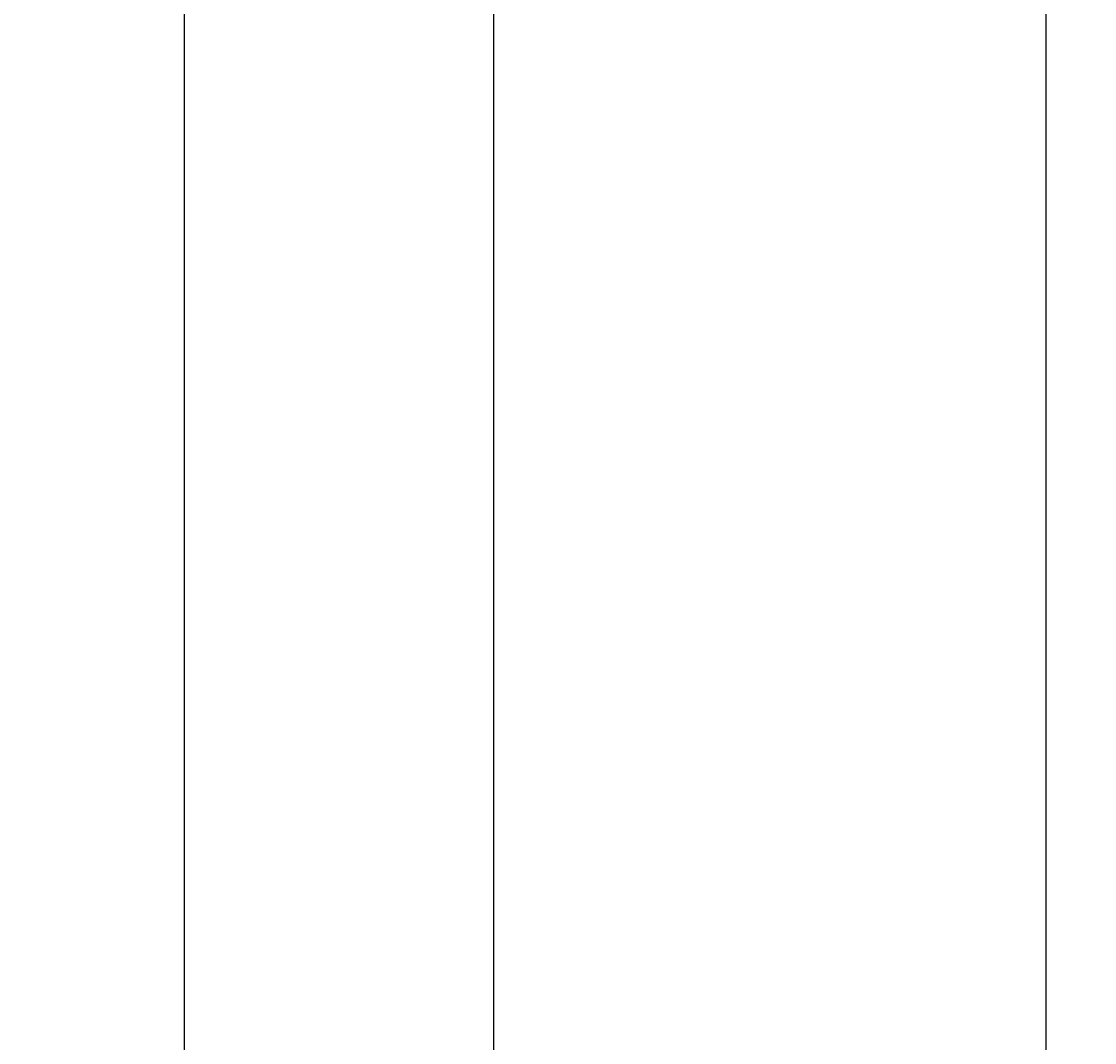
# Model space of a CAD drawing. Units: inches. Extents: x -61 to 1599, y -1316 to 257.
# Tile 77 of 204: x 240 to 323, y -565 to -486. Entities that reach past the tile are written whole.
import ezdxf

# ---------------------------------------------------------------- set-up
doc = ezdxf.new("R2010")
doc.units = ezdxf.units.IN
doc.header["$MEASUREMENT"] = 0
doc.layers.add('A-ANNO-DIMS', color=2, linetype='Continuous', lineweight=18)
doc.styles.get("Standard").update_dxf_attribs({"font": 'arial.ttf'})
doc.dimstyles.get("Standard").update_dxf_attribs({"dimtxt": 0.18, "dimasz": 0.18, "dimexe": 0.18, "dimexo": 0.0625, "dimgap": 0.09, "dimtad": 0, "dimtih": 1, "dimtoh": 1, "dimdec": 0, "dimzin": 0, "dimdsep": 46, "dimlunit": 3, "dimtxsty": 'Standard', "dimcen": 0.09, "dimadec": 0, "dimazin": 0, "dimtfac": 1, "dimtdec": 0, "dimtofl": 0, "dimtmove": 0, "dimatfit": 3, "dimfxl": 1, "dimtolj": 1, "dimtzin": 0, "dimarcsym": 0})

# ---------------------------------------------------------------- blocks, each defined once
blk = doc.blocks.new('*D687')
at = {"layer": 'A-ANNO-DIMS', "color": 0, "lineweight": -2, "transparency": 16777216}
for p, q in [((289.418, 181.677), (-61.077, 181.677)), ((-60.897, 181.497), (-60.897, -528.952)), ((-60.897, -1239.765), (-60.897, -529.316)), ((319.64, -1239.945), (-61.077, -1239.945))]:
    blk.add_line(p, q, dxfattribs=at)
at = {"layer": 'A-ANNO-DIMS', "color": 0, "transparency": 16777216}
for points in [[(-60.927, 181.497), (-60.867, 181.497), (-60.897, 181.677)], [(-60.927, -1239.765), (-60.867, -1239.765), (-60.897, -1239.945)]]:
    blk.add_solid(points, dxfattribs=at)
at = {"layer": 'DEFPOINTS', "color": 0, "transparency": 16777216}
for p in [(289.481, 181.677), (-60.897, -1239.945), (319.703, -1239.945)]:
    blk.add_point(p, dxfattribs=at)
at = {"layer": 'A-ANNO-DIMS', "color": 0, "transparency": 16777216, "insert": (-60.897, -529.134), "char_height": 0.18, "attachment_point": 5}
blk.add_mtext('\\A1;1421.6', dxfattribs=at)
blk = doc.blocks.new('*D701')
at = {"layer": 'A-ANNO-DIMS', "color": 0, "lineweight": -2, "transparency": 16777216}
for p, q in [((215.752, -616.882), (215.752, 257.457)), ((215.932, 257.277), (233.924, 257.277)), ((252.702, 257.277), (234.711, 257.277)), ((252.882, -616.882), (252.882, 257.457))]:
    blk.add_line(p, q, dxfattribs=at)
at = {"layer": 'A-ANNO-DIMS', "color": 0, "transparency": 16777216}
for points in [[(215.932, 257.307), (215.932, 257.247), (215.752, 257.277)], [(252.702, 257.307), (252.702, 257.247), (252.882, 257.277)]]:
    blk.add_solid(points, dxfattribs=at)
at = {"layer": 'DEFPOINTS', "color": 0, "transparency": 16777216}
for p in [(252.882, 257.277), (215.752, -616.945), (252.882, -616.945)]:
    blk.add_point(p, dxfattribs=at)
at = {"layer": 'A-ANNO-DIMS', "color": 0, "transparency": 16777216, "insert": (234.317, 257.277), "char_height": 0.18, "attachment_point": 5}
blk.add_mtext('\\A1;37.13', dxfattribs=at)
blk = doc.blocks.new('*D702')
at = {"layer": 'A-ANNO-DIMS', "color": 0, "lineweight": -2, "transparency": 16777216}
for p, q in [((276.882, -616.882), (276.882, 257.457)), ((277.062, 257.277), (312.209, 257.277)), ((348.14, 257.277), (312.994, 257.277)), ((348.32, -616.882), (348.32, 257.457))]:
    blk.add_line(p, q, dxfattribs=at)
at = {"layer": 'A-ANNO-DIMS', "color": 0, "transparency": 16777216}
for points in [[(277.062, 257.307), (277.062, 257.247), (276.882, 257.277)], [(348.14, 257.307), (348.14, 257.247), (348.32, 257.277)]]:
    blk.add_solid(points, dxfattribs=at)
at = {"layer": 'DEFPOINTS', "color": 0, "transparency": 16777216}
for p in [(348.32, 257.277), (276.882, -616.945), (348.32, -616.945)]:
    blk.add_point(p, dxfattribs=at)
at = {"layer": 'A-ANNO-DIMS', "color": 0, "transparency": 16777216, "insert": (312.601, 257.277), "char_height": 0.18, "attachment_point": 5}
blk.add_mtext('\\A1;71.44', dxfattribs=at)
blk = doc.blocks.new('*D710')
at = {"layer": 'A-ANNO-DIMS', "color": 0, "lineweight": -2, "transparency": 16777216}
for p, q in [((319.703, -465.385), (319.703, -1315.725)), ((403.703, -465.385), (403.703, -1315.725)), ((319.883, -1315.545), (361.484, -1315.545)), ((403.523, -1315.545), (361.921, -1315.545))]:
    blk.add_line(p, q, dxfattribs=at)
at = {"layer": 'A-ANNO-DIMS', "color": 0, "transparency": 16777216}
for points in [[(319.883, -1315.515), (319.883, -1315.575), (319.703, -1315.545)], [(403.523, -1315.515), (403.523, -1315.575), (403.703, -1315.545)]]:
    blk.add_solid(points, dxfattribs=at)
at = {"layer": 'DEFPOINTS', "color": 0, "transparency": 16777216}
for p in [(319.703, -465.323), (403.703, -465.323), (403.703, -1315.545)]:
    blk.add_point(p, dxfattribs=at)
at = {"layer": 'A-ANNO-DIMS', "color": 0, "transparency": 16777216, "insert": (361.703, -1315.545), "char_height": 0.18, "attachment_point": 5}
blk.add_mtext('\\A1;84', dxfattribs=at)

msp = doc.modelspace()

# ---------------------------------------------------------------- dimensions: what is measured, and where the dimension line sits
at = {"layer": 'A-ANNO-DIMS'}
for base, p1, p2, override, picture, middle in [((252.8825, 257.2771), (215.7521, -616.9446), (252.8825, -616.9446), {"dimdec": 2, "dimlfac": 1, "dimrnd": 0, "dimzin": 0, "dimdsep": 46, "dimlunit": 2}, '*D701', (234.3173, 257.2771)), ((348.3201, 257.2771), (276.8825, -616.9446), (348.3201, -616.9446), {"dimdec": 2, "dimlfac": 1, "dimrnd": 0, "dimzin": 0, "dimdsep": 46, "dimlunit": 2}, '*D702', (312.6013, 257.2771)), ((403.7028, -1315.5446), (319.7028, -465.3229), (403.7028, -465.3229), {"dimdec": 0, "dimlfac": 1, "dimrnd": 0, "dimzin": 0, "dimdsep": 46, "dimlunit": 2}, '*D710', (361.7028, -1315.5446))]:
    dim = msp.add_linear_dim(base=base, p1=p1, p2=p2, dimstyle='Standard', override=override, dxfattribs=at)
    dim.commit()
    dim.dimension.update_dxf_attribs({"geometry": picture, "text_midpoint": middle})
dim = msp.add_linear_dim(base=(-60.8972, -1239.9446), p1=(289.4807, 181.6771), p2=(319.7028, -1239.9446), angle=90, dimstyle='Standard', override={"dimdec": 1, "dimlfac": 1, "dimrnd": 0, "dimzin": 0, "dimdsep": 46, "dimlunit": 2}, dxfattribs=at)
dim.commit()
dim.dimension.update_dxf_attribs({"geometry": '*D687', "text_midpoint": (-60.8972, -529.1337)})

doc.saveas('drawing.dxf')
